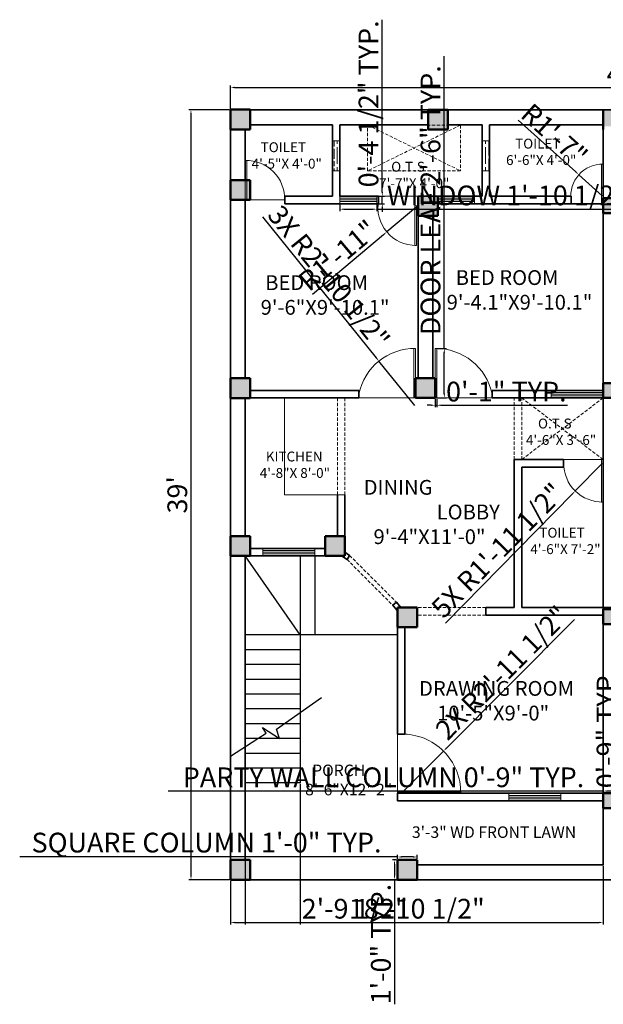
# Model space of a CAD drawing. Units: inches. Extents: x 2499 to 3266, y 1908 to 2597.
# Tile 1 of 2: x 2499 to 2854, y 1908 to 2507. Entities that reach past the tile are written whole.
import ezdxf

# ---------------------------------------------------------------- set-up
doc = ezdxf.new("R2010")
doc.units = ezdxf.units.IN
doc.linetypes.add('JIS_02_2.0', pattern=[3, 2, -1])
for name, color, linetype, lineweight in [('A-ANNO-DIMS', 2, 'Continuous', 18), ('A-AREA-IDEN', 7, 'Continuous', 18), ('A-COLS', 7, 'Continuous', 50), ('A-FLOR-FIXT', 9, 'Continuous', 18), ('A-FLOR-OPEN', 6, 'JIS_02_2.0', 13), ('A-FLOR-STRS', 7, 'Continuous', 25), ('A-GLAZ', 5, 'Continuous', 18), ('A-GLAZ-PATT', 4, 'Continuous', 13), ('A-WALL', 7, 'Continuous', 35), ('A-WALL-OVHD', 6, 'JIS_02_2.0', 18)]:
    doc.layers.add(name, color=color, linetype=linetype, lineweight=lineweight)
doc.layers.add('A-COLS-PATT', color=177, linetype='Continuous', lineweight=13, true_color=0x293189)
doc.layers.add('A-DOOR', color=32, linetype='Continuous', lineweight=18, true_color=0xcd6928)
doc.styles.get("Standard").update_dxf_attribs({"font": 'arial.ttf'})
doc.dimstyles.new('ISO-25', dxfattribs={"dimtxt": 12, "dimasz": 2.5, "dimexe": 1.25, "dimexo": 0.625, "dimtad": 1, "dimdec": 1, "dimlunit": 3, "dimtxsty": 'Standard', "dimcen": 2.5, "dimadec": 0, "dimazin": 0, "dimtfac": 1, "dimtdec": 1, "dimtmove": 0, "dimatfit": 3, "dimfxl": 1, "dimarcsym": 0})

# ---------------------------------------------------------------- blocks, each defined once
blk = doc.blocks.new('*D4')
at = {"layer": 'A-ANNO-DIMS', "color": 0, "lineweight": -2, "transparency": 16777216}
for p, q in [((2627.06, 2452.33), (2627.06, 2466.64)), ((3107.06, 2452.33), (3107.06, 2466.64)), ((2629.56, 2465.39), (3104.56, 2465.39))]:
    blk.add_line(p, q, dxfattribs=at)
at = {"layer": 'A-ANNO-DIMS', "color": 0, "transparency": 16777216}
for points in [[(2629.56, 2465.81), (2629.56, 2464.98), (2627.06, 2465.39)], [(3104.56, 2465.81), (3104.56, 2464.98), (3107.06, 2465.39)]]:
    blk.add_solid(points, dxfattribs=at)
at = {"layer": 'Defpoints', "color": 0, "transparency": 16777216}
for p in [(3107.06, 2465.39), (2627.06, 2451.71), (3107.06, 2451.71)]:
    blk.add_point(p, dxfattribs=at)
at = {"layer": 'A-ANNO-DIMS', "color": 0, "transparency": 16777216, "insert": (2867.06, 2472.14), "char_height": 12, "attachment_point": 5}
blk.add_mtext("40'", dxfattribs=at)
blk = doc.blocks.new('*D5')
at = {"layer": 'A-ANNO-DIMS', "color": 0, "lineweight": -2, "transparency": 16777216}
for p, q in [((2626.43, 2451.71), (2601.81, 2451.71)), ((2603.06, 2449.21), (2603.06, 1986.21)), ((2626.43, 1983.71), (2601.81, 1983.71))]:
    blk.add_line(p, q, dxfattribs=at)
at = {"layer": 'A-ANNO-DIMS', "color": 0, "transparency": 16777216}
for points in [[(2602.64, 2449.21), (2603.48, 2449.21), (2603.06, 2451.71)], [(2602.64, 1986.21), (2603.48, 1986.21), (2603.06, 1983.71)]]:
    blk.add_solid(points, dxfattribs=at)
at = {"layer": 'Defpoints', "color": 0, "transparency": 16777216}
for p in [(2627.06, 2451.71), (2603.06, 1983.71), (2627.06, 1983.71)]:
    blk.add_point(p, dxfattribs=at)
at = {"layer": 'A-ANNO-DIMS', "color": 0, "transparency": 16777216, "insert": (2596.3, 2217.71), "char_height": 12, "attachment_point": 5, "rotation": 90}
blk.add_mtext("39'", dxfattribs=at)
blk = doc.blocks.new('COL-12X12')
for p, q in [((0, 12), (12, 12)), ((0, 0), (0, 12)), ((12, 12), (12, 0)), ((12, 0), (0, 0))]:
    blk.add_line(p, q)
blk = doc.blocks.new('COL-9X9')
for p, q in [((0, 9), (9, 9)), ((0, 0), (0, 9)), ((9, 9), (9, 0)), ((9, 0), (0, 0))]:
    blk.add_line(p, q)
blk = doc.blocks.new('WIN-31_54')
for p, q in [((0, 4.5), (0, 0)), ((0, 3.25), (31.54, 3.25)), ((0, 2.25), (31.54, 2.25)), ((0, 1.25), (31.54, 1.25)), ((31.54, 0), (31.54, 4.5)), ((31.54, 3.25), (31.54, 0))]:
    blk.add_line(p, q)
blk = doc.blocks.new('WIN-22_41')
for p, q in [((0, 4.5), (0, 0)), ((22.41, 3.25), (0, 3.25)), ((22.41, 2.25), (0, 2.25)), ((22.41, 1.25), (0, 1.25)), ((22.41, 4.5), (22.41, 0))]:
    blk.add_line(p, q)
blk = doc.blocks.new('STAIR-BREAK')
for p, q in [((28.01, 16.3), (55.25, 35.7)), ((16.69, 10.65), (21.73, 13.87)), ((21.73, 13.87), (19.46, 17.43)), ((19.46, 17.43), (29.77, 10.65)), ((29.77, 10.65), (28.01, 16.3)), ((0, 0), (16.69, 10.65))]:
    blk.add_line(p, q)
blk = doc.blocks.new('OTS-REAR-OPENING')
for p, q in [((0, 27.82), (56.41, 0)), ((56.41, 27.82), (0, 0))]:
    blk.add_line(p, q)
blk.add_lwpolyline([(0, 27.82), (56.41, 27.82), (56.41, 0), (0, 0)], close=True)
blk = doc.blocks.new('DOOR-LEAF-24')
for p, q in [((0, 0), (0, 24)), ((0, 24), (1, 24)), ((1, 24), (1, 0)), ((1, 0), (0, 0))]:
    blk.add_line(p, q)
blk = doc.blocks.new('DOOR-LEAF-30')
for p, q in [((0, 6), (0, 30)), ((0, 30), (1, 30)), ((1, 30), (1, 0)), ((1, 0), (0, 0))]:
    blk.add_line(p, q)
blk = doc.blocks.new('*D14')
at = {"layer": 'A-ANNO-DIMS', "color": 0, "lineweight": -2, "transparency": 16777216}
for p, q in [((2728.56, 1997.51), (2498.96, 1997.51)), ((2728.56, 1996.33), (2728.56, 1998.76)), ((2738.06, 1997.51), (2731.06, 1997.51)), ((2740.56, 1996.33), (2740.56, 1998.76))]:
    blk.add_line(p, q, dxfattribs=at)
at = {"layer": 'A-ANNO-DIMS', "color": 0, "transparency": 16777216}
for points in [[(2731.06, 1997.93), (2731.06, 1997.09), (2728.56, 1997.51)], [(2738.06, 1997.93), (2738.06, 1997.09), (2740.56, 1997.51)]]:
    blk.add_solid(points, dxfattribs=at)
at = {"layer": 'Defpoints', "color": 0, "transparency": 16777216}
for p in [(2728.56, 1997.51), (2728.56, 1995.71), (2740.56, 1995.71)]:
    blk.add_point(p, dxfattribs=at)
at = {"layer": 'A-ANNO-DIMS', "color": 0, "transparency": 16777216, "insert": (2612.51, 2004.71), "char_height": 12, "attachment_point": 5}
blk.add_mtext('SQUARE COLUMN 1\'-0" TYP.', dxfattribs=at)
blk = doc.blocks.new('*D15')
at = {"layer": 'A-ANNO-DIMS', "color": 0, "lineweight": -2, "transparency": 16777216}
for p, q in [((2727.93, 1995.71), (2725.51, 1995.71)), ((2726.76, 1993.21), (2726.76, 1986.21)), ((2727.93, 1983.71), (2725.51, 1983.71)), ((2726.76, 1983.71), (2726.76, 1907.94))]:
    blk.add_line(p, q, dxfattribs=at)
at = {"layer": 'A-ANNO-DIMS', "color": 0, "transparency": 16777216}
for points in [[(2726.34, 1993.21), (2727.17, 1993.21), (2726.76, 1995.71)], [(2726.34, 1986.21), (2727.17, 1986.21), (2726.76, 1983.71)]]:
    blk.add_solid(points, dxfattribs=at)
at = {"layer": 'Defpoints', "color": 0, "transparency": 16777216}
for p in [(2728.56, 1995.71), (2726.76, 1983.71), (2728.56, 1983.71)]:
    blk.add_point(p, dxfattribs=at)
at = {"layer": 'A-ANNO-DIMS', "color": 0, "transparency": 16777216, "insert": (2720.01, 1944.58), "char_height": 12, "attachment_point": 5, "rotation": 90}
blk.add_mtext('1\'-0" TYP.', dxfattribs=at)
blk = doc.blocks.new('*D16')
at = {"layer": 'A-ANNO-DIMS', "color": 0, "lineweight": -2, "transparency": 16777216}
for p, q in [((2853.56, 2037.57), (2589.1, 2037.57)), ((2853.56, 2036.85), (2853.56, 2038.82)), ((2860.06, 2037.57), (2856.06, 2037.57)), ((2862.56, 2036.85), (2862.56, 2038.82))]:
    blk.add_line(p, q, dxfattribs=at)
at = {"layer": 'A-ANNO-DIMS', "color": 0, "transparency": 16777216}
for points in [[(2856.06, 2037.99), (2856.06, 2037.15), (2853.56, 2037.57)], [(2860.06, 2037.99), (2860.06, 2037.15), (2862.56, 2037.57)]]:
    blk.add_solid(points, dxfattribs=at)
at = {"layer": 'Defpoints', "color": 0, "transparency": 16777216}
for p in [(2853.56, 2037.57), (2853.56, 2036.22), (2862.56, 2036.22)]:
    blk.add_point(p, dxfattribs=at)
at = {"layer": 'A-ANNO-DIMS', "color": 0, "transparency": 16777216, "insert": (2720.08, 2044.4), "char_height": 12, "attachment_point": 5}
blk.add_mtext('PARTY WALL COLUMN 0\'-9" TYP.', dxfattribs=at)
blk = doc.blocks.new('*D17')
at = {"layer": 'A-ANNO-DIMS', "color": 0, "lineweight": -2, "transparency": 16777216}
for p, q in [((2863.91, 2036.22), (2863.91, 2113.12)), ((2863.18, 2036.22), (2865.16, 2036.22)), ((2863.91, 2029.72), (2863.91, 2033.72)), ((2863.18, 2027.22), (2865.16, 2027.22))]:
    blk.add_line(p, q, dxfattribs=at)
at = {"layer": 'A-ANNO-DIMS', "color": 0, "transparency": 16777216}
for points in [[(2863.49, 2033.72), (2864.32, 2033.72), (2863.91, 2036.22)], [(2863.49, 2029.72), (2864.32, 2029.72), (2863.91, 2027.22)]]:
    blk.add_solid(points, dxfattribs=at)
at = {"layer": 'Defpoints', "color": 0, "transparency": 16777216}
for p in [(2862.56, 2036.22), (2863.91, 2036.22), (2862.56, 2027.22)]:
    blk.add_point(p, dxfattribs=at)
at = {"layer": 'A-ANNO-DIMS', "color": 0, "transparency": 16777216, "insert": (2857.16, 2075.92), "char_height": 12, "attachment_point": 5, "rotation": 90}
blk.add_mtext('0\'-9" TYP.', dxfattribs=at)
blk = doc.blocks.new('*D20')
at = {"layer": 'A-ANNO-DIMS', "color": 0, "lineweight": -2, "transparency": 16777216}
for p, q in [((2693.56, 2394.08), (2693.56, 2390.1)), ((2696.06, 2391.35), (2713.47, 2391.35)), ((2715.97, 2394.08), (2715.97, 2390.1)), ((2715.97, 2391.35), (2908.86, 2391.35))]:
    blk.add_line(p, q, dxfattribs=at)
at = {"layer": 'A-ANNO-DIMS', "color": 0, "transparency": 16777216}
for points in [[(2696.06, 2391.76), (2696.06, 2390.93), (2693.56, 2391.35)], [(2713.47, 2391.76), (2713.47, 2390.93), (2715.97, 2391.35)]]:
    blk.add_solid(points, dxfattribs=at)
at = {"layer": 'Defpoints', "color": 0, "transparency": 16777216}
for p in [(2693.56, 2394.71), (2715.97, 2394.71), (2715.97, 2391.35)]:
    blk.add_point(p, dxfattribs=at)
at = {"layer": 'A-ANNO-DIMS', "color": 0, "transparency": 16777216, "insert": (2813.66, 2398.18), "char_height": 12, "attachment_point": 5}
blk.add_mtext('WINDOW 1\'-10 1/2" TYP.', dxfattribs=at)
blk = doc.blocks.new('*D21')
at = {"layer": 'A-ANNO-DIMS', "color": 0, "lineweight": -2, "transparency": 16777216}
for p, q in [((2719.33, 2401.71), (2719.33, 2506.57)), ((2716.6, 2399.21), (2720.58, 2399.21)), ((2716.6, 2394.71), (2720.58, 2394.71)), ((2719.33, 2394.71), (2719.33, 2399.21)), ((2719.33, 2392.21), (2719.33, 2389.71))]:
    blk.add_line(p, q, dxfattribs=at)
at = {"layer": 'A-ANNO-DIMS', "color": 0, "transparency": 16777216}
for points in [[(2718.92, 2401.71), (2719.75, 2401.71), (2719.33, 2399.21)], [(2718.92, 2392.21), (2719.75, 2392.21), (2719.33, 2394.71)]]:
    blk.add_solid(points, dxfattribs=at)
at = {"layer": 'Defpoints', "color": 0, "transparency": 16777216}
for p in [(2715.97, 2399.21), (2715.97, 2394.71), (2719.33, 2399.21)]:
    blk.add_point(p, dxfattribs=at)
at = {"layer": 'A-ANNO-DIMS', "color": 0, "transparency": 16777216, "insert": (2712.5, 2455.39), "char_height": 12, "attachment_point": 5, "rotation": 90}
blk.add_mtext('0\'-4 1/2" TYP.', dxfattribs=at)
blk = doc.blocks.new('*D24')
at = {"layer": 'A-ANNO-DIMS', "color": 0, "lineweight": -2, "transparency": 16777216}
for p, q in [((2757.02, 2306.66), (2757.02, 2484.49)), ((2753.15, 2306.66), (2758.27, 2306.66)), ((2757.02, 2279.16), (2757.02, 2304.16)), ((2753.15, 2276.66), (2758.27, 2276.66))]:
    blk.add_line(p, q, dxfattribs=at)
at = {"layer": 'A-ANNO-DIMS', "color": 0, "transparency": 16777216}
for points in [[(2756.6, 2304.16), (2757.44, 2304.16), (2757.02, 2306.66)], [(2756.6, 2279.16), (2757.44, 2279.16), (2757.02, 2276.66)]]:
    blk.add_solid(points, dxfattribs=at)
at = {"layer": 'Defpoints', "color": 0, "transparency": 16777216}
for p in [(2752.52, 2306.66), (2757.02, 2306.66), (2752.52, 2276.66)]:
    blk.add_point(p, dxfattribs=at)
at = {"layer": 'A-ANNO-DIMS', "color": 0, "transparency": 16777216, "insert": (2750.19, 2396.83), "char_height": 12, "attachment_point": 5, "rotation": 90}
blk.add_mtext('DOOR LEAF 2\'-6" TYP.', dxfattribs=at)
blk = doc.blocks.new('*D25')
at = {"layer": 'A-ANNO-DIMS', "color": 0, "lineweight": -2, "transparency": 16777216}
for p, q in [((2751.52, 2276.04), (2751.52, 2270.91)), ((2752.52, 2276.04), (2752.52, 2270.91)), ((2749.02, 2272.16), (2746.52, 2272.16)), ((2751.52, 2272.16), (2752.52, 2272.16)), ((2755.02, 2272.16), (2831.92, 2272.16))]:
    blk.add_line(p, q, dxfattribs=at)
at = {"layer": 'A-ANNO-DIMS', "color": 0, "transparency": 16777216}
for points in [[(2749.02, 2272.58), (2749.02, 2271.75), (2751.52, 2272.16)], [(2755.02, 2272.58), (2755.02, 2271.75), (2752.52, 2272.16)]]:
    blk.add_solid(points, dxfattribs=at)
at = {"layer": 'Defpoints', "color": 0, "transparency": 16777216}
for p in [(2751.52, 2276.66), (2752.52, 2276.66), (2752.52, 2272.16)]:
    blk.add_point(p, dxfattribs=at)
at = {"layer": 'A-ANNO-DIMS', "color": 0, "transparency": 16777216, "insert": (2794.72, 2278.91), "char_height": 12, "attachment_point": 5}
blk.add_mtext('0\'-1" TYP.', dxfattribs=at)
blk = doc.blocks.new('*D28')
at = {"layer": 'A-ANNO-DIMS', "color": 0, "lineweight": -2, "transparency": 16777216}
for p, q in [((2853.56, 1992.08), (2853.56, 1956.43)), ((2627.06, 1983.08), (2627.06, 1956.43)), ((2629.56, 1957.68), (2851.06, 1957.68))]:
    blk.add_line(p, q, dxfattribs=at)
at = {"layer": 'A-ANNO-DIMS', "color": 0, "transparency": 16777216}
for points in [[(2629.56, 1958.1), (2629.56, 1957.27), (2627.06, 1957.68)], [(2851.06, 1958.1), (2851.06, 1957.27), (2853.56, 1957.68)]]:
    blk.add_solid(points, dxfattribs=at)
at = {"layer": 'Defpoints', "color": 0, "transparency": 16777216}
for p in [(2853.56, 1992.71), (2627.06, 1983.71), (2853.56, 1957.68)]:
    blk.add_point(p, dxfattribs=at)
at = {"layer": 'A-ANNO-DIMS', "color": 0, "transparency": 16777216, "insert": (2740.31, 1964.51), "char_height": 12, "attachment_point": 5}
blk.add_mtext('18\'-10 1/2"', dxfattribs=at)
blk = doc.blocks.new('*D31')
at = {"layer": 'A-ANNO-DIMS', "color": 0, "lineweight": -2, "transparency": 16777216}
for p, q in [((2636.06, 2041.89), (2636.06, 1956.43)), ((2669.43, 2041.89), (2669.43, 1956.43)), ((2638.56, 1957.68), (2666.93, 1957.68)), ((2669.43, 1957.68), (2733.24, 1957.68))]:
    blk.add_line(p, q, dxfattribs=at)
at = {"layer": 'A-ANNO-DIMS', "color": 0, "transparency": 16777216}
for points in [[(2638.56, 1958.1), (2638.56, 1957.27), (2636.06, 1957.68)], [(2666.93, 1958.1), (2666.93, 1957.27), (2669.43, 1957.68)]]:
    blk.add_solid(points, dxfattribs=at)
at = {"layer": 'Defpoints', "color": 0, "transparency": 16777216}
for p in [(2636.06, 2042.51), (2669.43, 2042.51), (2669.43, 1957.68)]:
    blk.add_point(p, dxfattribs=at)
at = {"layer": 'A-ANNO-DIMS', "color": 0, "transparency": 16777216, "insert": (2702.58, 1964.51), "char_height": 12, "attachment_point": 5}
blk.add_mtext('2\'-9 1/2"', dxfattribs=at)
blk = doc.blocks.new('*D34')
at = {"layer": 'A-ANNO-DIMS', "color": 0, "lineweight": -2, "transparency": 16777216}
for p, q in [((2836.17, 2141.9), (2758.28, 2063.65)), ((2731.47, 2036.71), (2756.52, 2061.87))]:
    blk.add_line(p, q, dxfattribs=at)
at = {"layer": 'A-ANNO-DIMS', "color": 0, "transparency": 16777216}
blk.add_solid([(2757.99, 2063.94), (2758.58, 2063.35), (2756.52, 2061.87)], dxfattribs=at)
at = {"layer": 'Defpoints', "color": 0, "transparency": 16777216}
for p in [(2756.52, 2061.87), (2731.47, 2036.71)]:
    blk.add_point(p, dxfattribs=at)
at = {"layer": 'A-ANNO-DIMS', "color": 0, "transparency": 16777216, "insert": (2793.27, 2108.48), "char_height": 12, "attachment_point": 5, "rotation": 45.13418}
blk.add_mtext('2X R2\'-11 1/2"', dxfattribs=at)
blk = doc.blocks.new('*D36')
at = {"layer": 'A-ANNO-DIMS', "color": 0, "lineweight": -2, "transparency": 16777216}
for p, q in [((2646.51, 2386.7), (2715.7, 2300.93)), ((2739.02, 2272.02), (2717.27, 2298.99))]:
    blk.add_line(p, q, dxfattribs=at)
at = {"layer": 'A-ANNO-DIMS', "color": 0, "transparency": 16777216}
blk.add_solid([(2716.02, 2301.19), (2715.37, 2300.67), (2717.27, 2298.99)], dxfattribs=at)
at = {"layer": 'Defpoints', "color": 0, "transparency": 16777216}
for p in [(2717.27, 2298.99), (2739.02, 2272.02)]:
    blk.add_point(p, dxfattribs=at)
at = {"layer": 'A-ANNO-DIMS', "color": 0, "transparency": 16777216, "insert": (2685.64, 2349.08), "char_height": 12, "attachment_point": 5, "rotation": 308.89333}
blk.add_mtext('3X R2\'-10 1/2"', dxfattribs=at)
blk = doc.blocks.new('*D37')
at = {"layer": 'A-ANNO-DIMS', "color": 0, "lineweight": -2, "transparency": 16777216}
for p, q in [((2853.06, 2236.82), (2836.6, 2220.04)), ((2757.7, 2139.57), (2834.85, 2218.26))]:
    blk.add_line(p, q, dxfattribs=at)
at = {"layer": 'A-ANNO-DIMS', "color": 0, "transparency": 16777216}
blk.add_solid([(2834.56, 2218.55), (2835.15, 2217.96), (2836.6, 2220.04)], dxfattribs=at)
at = {"layer": 'Defpoints', "color": 0, "transparency": 16777216}
for p in [(2853.06, 2236.82), (2836.6, 2220.04)]:
    blk.add_point(p, dxfattribs=at)
at = {"layer": 'A-ANNO-DIMS', "color": 0, "transparency": 16777216, "insert": (2790.52, 2182.8), "char_height": 12, "attachment_point": 5, "rotation": 45.56344}
blk.add_mtext('5X R1\'-11 1/2"', dxfattribs=at)
blk = doc.blocks.new('*D38')
at = {"layer": 'A-ANNO-DIMS', "color": 0, "lineweight": -2, "transparency": 16777216}
for p, q in [((2739.74, 2392.38), (2722.06, 2377.53)), ((2676.92, 2339.61), (2720.15, 2375.92))]:
    blk.add_line(p, q, dxfattribs=at)
at = {"layer": 'A-ANNO-DIMS', "color": 0, "transparency": 16777216}
blk.add_solid([(2719.88, 2376.24), (2720.42, 2375.6), (2722.06, 2377.53)], dxfattribs=at)
at = {"layer": 'Defpoints', "color": 0, "transparency": 16777216}
for p in [(2739.74, 2392.38), (2722.06, 2377.53)]:
    blk.add_point(p, dxfattribs=at)
at = {"layer": 'A-ANNO-DIMS', "color": 0, "transparency": 16777216, "insert": (2693.3, 2362.05), "char_height": 12, "attachment_point": 5, "rotation": 40.03317}
blk.add_mtext('R1\'-11"', dxfattribs=at)
blk = doc.blocks.new('*D40')
at = {"layer": 'A-ANNO-DIMS', "color": 0, "lineweight": -2, "transparency": 16777216}
for p, q in [((2801.82, 2445.47), (2836.92, 2414.01)), ((2853.06, 2399.54), (2838.78, 2412.34))]:
    blk.add_line(p, q, dxfattribs=at)
at = {"layer": 'A-ANNO-DIMS', "color": 0, "transparency": 16777216}
blk.add_solid([(2837.2, 2414.32), (2836.64, 2413.7), (2838.78, 2412.34)], dxfattribs=at)
at = {"layer": 'Defpoints', "color": 0, "transparency": 16777216}
for p in [(2838.78, 2412.34), (2853.06, 2399.54)]:
    blk.add_point(p, dxfattribs=at)
at = {"layer": 'A-ANNO-DIMS', "color": 0, "transparency": 16777216, "insert": (2822.88, 2435.53), "char_height": 12, "attachment_point": 5, "rotation": 318.12284}
blk.add_mtext('R1\'-7"', dxfattribs=at)

msp = doc.modelspace()

# ---------------------------------------------------------------- hatches: boundary and pattern name
at = {"layer": 'A-COLS-PATT'}
h = msp.add_hatch(color=256, dxfattribs=at)
h.dxf.hatch_style = 1
h.paths.add_polyline_path([(2639.06, 2451.71), (2627.06, 2451.71), (2627.06, 2439.9), (2639.06, 2439.9)])
h.paths.add_polyline_path([(2639.06, 2408.96), (2627.06, 2408.96), (2627.06, 2396.96), (2639.06, 2396.96)])
h.paths.add_polyline_path([(2759.22, 2451.71), (2747.22, 2451.71), (2747.22, 2439.71), (2759.22, 2439.71)])
h.paths.add_polyline_path([(2862.56, 2451.71), (2853.74, 2451.71), (2853.56, 2451.71), (2853.56, 2441.73), (2853.74, 2441.73), (2853.74, 2441.73), (2862.56, 2441.73), (2862.56, 2442.71)])
h.paths.add_polyline_path([(2989.26, 2451.71), (2977.26, 2451.71), (2977.26, 2439.71), (2989.26, 2439.71)])
h.paths.add_polyline_path([(3107.06, 2451.71), (3095.06, 2451.71), (3095.06, 2439.71), (3107.06, 2439.71)])
h.paths.add_polyline_path([(3107.06, 2399.21), (3095.06, 2399.21), (3095.06, 2387.21), (3107.06, 2387.21)])
h.paths.add_polyline_path([(2989.26, 2399.21), (2977.26, 2399.21), (2977.26, 2387.21), (2989.26, 2387.21)])
h.paths.add_polyline_path([(2862.56, 2397.96), (2853.56, 2397.96), (2853.56, 2388.96), (2862.56, 2388.96)])
h.paths.add_polyline_path([(2753.06, 2399.21), (2741.06, 2399.21), (2741.06, 2387.39), (2753.06, 2387.39)])
h.paths.add_polyline_path([(2639.06, 2288.56), (2627.06, 2288.56), (2627.06, 2276.56), (2636.06, 2276.56), (2636.06, 2276.61), (2639.06, 2276.61)])
h.paths.add_polyline_path([(2862.56, 2285.61), (2853.56, 2285.61), (2853.56, 2276.61), (2862.56, 2276.61)])
h.paths.add_polyline_path([(2990.61, 2288.63), (2978.61, 2288.63), (2978.61, 2276.63), (2990.61, 2276.63)])
h.paths.add_polyline_path([(3107.06, 2288.61), (3095.06, 2288.61), (3095.06, 2276.61), (3107.06, 2276.61)])
h.paths.add_polyline_path([(3107.06, 2192.61), (3095.06, 2192.61), (3095.06, 2180.61), (3107.06, 2180.61)])
h.paths.add_polyline_path([(3045.56, 2192.61), (3033.56, 2192.61), (3033.56, 2180.61), (3045.56, 2180.61)])
h.paths.add_polyline_path([(2639.06, 2192.61), (2627.06, 2192.61), (2627.06, 2180.61), (2639.06, 2180.61)])
h.paths.add_polyline_path([(2696.54, 2192.61), (2684.54, 2192.61), (2684.54, 2180.61), (2696.54, 2180.61)])
h.paths.add_polyline_path([(2740.56, 2149.11), (2728.56, 2149.11), (2728.56, 2137.17), (2740.56, 2137.17)])
h.paths.add_polyline_path([(2862.56, 2148.12), (2853.56, 2148.12), (2853.56, 2139.12), (2862.56, 2139.12)])
h.paths.add_polyline_path([(2987.56, 2149.11), (2975.54, 2149.11), (2975.54, 2137.05), (2987.56, 2137.05)])
h.paths.add_polyline_path([(2862.56, 2036.21), (2853.56, 2036.21), (2853.56, 2027.22), (2862.56, 2027.22)])
h.paths.add_polyline_path([(2639.06, 1995.71), (2627.06, 1995.71), (2627.06, 1983.71), (2639.06, 1983.71)])
h.paths.add_polyline_path([(2740.56, 1995.71), (2728.56, 1995.71), (2728.56, 1983.71), (2740.56, 1983.71)])
h.paths.add_polyline_path([(2987.56, 1995.71), (2975.56, 1995.71), (2975.56, 1983.71), (2987.56, 1983.71)])
h.paths.add_polyline_path([(3107.06, 1995.71), (3095.06, 1995.71), (3095.06, 1983.71), (3107.06, 1983.71)])
h = msp.add_hatch(color=256, dxfattribs=at)
h.dxf.hatch_style = 1
h.paths.add_polyline_path([(2751.52, 2288.66), (2739.52, 2288.66), (2739.52, 2276.66), (2751.52, 2276.66)])
at = {"layer": 'A-GLAZ-PATT'}
h = msp.add_hatch(dxfattribs=at)
h.set_pattern_fill('GOST_WOOD', color=256)
h.paths.add_polyline_path([(2693.56, 2432.95), (2689.06, 2432.95), (2689.06, 2414.75), (2693.56, 2414.75)])
h.paths.add_polyline_path([(2784.56, 2432.95), (2780.06, 2432.95), (2780.06, 2414.75), (2784.56, 2414.75)])
h.paths.add_polyline_path([(2940.56, 2432.95), (2936.06, 2432.95), (2936.06, 2414.75), (2940.56, 2414.75)])
h.paths.add_polyline_path([(3031.56, 2432.95), (3027.06, 2432.95), (3027.06, 2414.75), (3031.56, 2414.75)])

# ---------------------------------------------------------------- linework, layer by layer
at = {"layer": 'A-COLS'}
for p, q in [((2853.56, 2439.71), (2853.56, 2451.71)), ((2853.74, 2441.73), (2853.56, 2441.73)), ((2741.06, 2387.39), (2741.06, 2399.21)), ((2753.06, 2399.21), (2753.06, 2387.39)), ((2753.06, 2387.39), (2741.06, 2387.39)), ((2636.06, 2180.61), (2627.06, 2180.61)), ((2728.56, 2149.11), (2740.56, 2149.11)), ((2728.56, 2137.17), (2728.56, 2149.11)), ((2740.56, 2149.11), (2740.56, 2137.17)), ((2740.56, 2137.17), (2728.56, 2137.17)), ((2728.56, 1995.71), (2728.56, 1983.71))]:
    msp.add_line(p, q, dxfattribs=at)
at = {"layer": 'A-DOOR'}
for p, q in [((2636.06, 2396.96), (2636.06, 2420.96)), ((2636.06, 2420.96), (2637.06, 2420.96)), ((2637.06, 2420.96), (2637.06, 2396.96)), ((2660.06, 2396.96), (2636.06, 2396.96)), ((2717.06, 2399.21), (2741.06, 2399.21)), ((2834.06, 2394.71), (2852.56, 2394.71)), ((2741.06, 2393.3), (2740.06, 2393.3)), ((2739.52, 2306.66), (2738.52, 2306.66)), ((2738.52, 2306.66), (2738.57, 2276.66)), ((2739.52, 2282.66), (2739.52, 2306.66)), ((2738.52, 2276.66), (2705.06, 2276.61)), ((2738.52, 2276.66), (2739.52, 2276.66)), ((2752.52, 2276.66), (2786.06, 2276.61)), ((2853.56, 2239.11), (2829.56, 2239.11)), ((2852.56, 2213.33), (2852.56, 2239.11)), ((2852.56, 2239.11), (2853.56, 2239.11)), ((2853.56, 2237.33), (2853.56, 2213.33)), ((2853.56, 2213.33), (2852.56, 2213.33)), ((2728.56, 2036.21), (2728.56, 2072.21)), ((2730.98, 2037.21), (2728.56, 2037.21)), ((2728.56, 2037.21), (2728.56, 2036.21)), ((2754.98, 2037.21), (2730.98, 2037.21)), ((2730.98, 2036.21), (2754.98, 2036.21)), ((2754.98, 2036.21), (2754.98, 2037.21)), ((2766.98, 2037.21), (2754.98, 2037.21)), ((2754.98, 2036.21), (2766.98, 2036.21)), ((2766.98, 2036.21), (2766.98, 2037.21))]:
    msp.add_line(p, q, dxfattribs=at)
for centre, radius, start, end in [((2636.56, 2397.46), 23.51, 358.78112, 91.21888), ((2853.06, 2399.54), 19.17, 88.50578, 187.73848), ((2739.74, 2392.38), 23.08, 169.27414, 270.79204), ((2739.02, 2272.02), 34.65, 89.1731, 168.61507), ((2752.02, 2271.93), 34.73, 11.50222, 90.82483), ((2853.06, 2236.82), 23.5, 179.90805, 271.21915), ((2731.47, 2036.71), 35.51, 359.19313, 91.07497)]:
    msp.add_arc(centre, radius, start, end, dxfattribs=at)
at = {"layer": 'A-FLOR-FIXT'}
for p, q in [((2659.83, 2217.63), (2659.83, 2276.61)), ((2696.56, 2217.63), (2659.83, 2217.63))]:
    msp.add_line(p, q, dxfattribs=at)
at = {"layer": 'A-FLOR-OPEN'}
for p, q in [((2710.42, 2414.75), (2710.56, 2414.75)), ((2766.7, 2414.75), (2766.84, 2414.75)), ((2799.56, 2239.11), (2799.56, 2276.61)), ((2804.06, 2239.11), (2804.06, 2276.61)), ((2853.56, 2276.61), (2804.06, 2239.11)), ((2804.06, 2239.11), (2804.06, 2276.61)), ((2804.06, 2276.61), (2853.56, 2239.11))]:
    msp.add_line(p, q, dxfattribs=at)
at = {"layer": 'A-FLOR-STRS'}
for p, q in [((2669.43, 2132.51), (2636.06, 2180.61)), ((2669.43, 2180.61), (2669.43, 2042.51)), ((2678.43, 2180.61), (2678.43, 2132.51)), ((2728.56, 2132.51), (2636.06, 2132.51)), ((2669.43, 2132.51), (2669.43, 2123.51)), ((2669.43, 2123.51), (2636.06, 2123.51)), ((2669.43, 2114.51), (2636.06, 2114.51)), ((2669.43, 2105.51), (2636.06, 2105.51)), ((2669.43, 2096.51), (2636.06, 2096.51)), ((2669.43, 2087.51), (2636.06, 2087.51)), ((2669.43, 2078.51), (2636.06, 2078.51)), ((2669.43, 2069.51), (2636.06, 2069.51)), ((2669.43, 2060.51), (2636.06, 2060.51)), ((2669.43, 2051.51), (2636.06, 2051.51)), ((2669.43, 2042.51), (2636.06, 2042.51))]:
    msp.add_line(p, q, dxfattribs=at)
at = {"layer": 'A-GLAZ'}
for p, q in [((2689.06, 2432.95), (2693.56, 2432.95)), ((2689.06, 2414.75), (2689.06, 2432.95)), ((2693.56, 2432.95), (2693.56, 2414.75)), ((2780.06, 2432.95), (2784.56, 2432.95)), ((2693.56, 2414.75), (2689.06, 2414.75)), ((2780.06, 2414.75), (2784.56, 2414.75)), ((2822.02, 2281.11), (2822.02, 2276.61)), ((2822.02, 2279.86), (2853.56, 2279.86)), ((2822.02, 2278.86), (2853.56, 2278.86)), ((2822.02, 2277.86), (2853.56, 2277.86))]:
    msp.add_line(p, q, dxfattribs=at)
at = {"layer": 'A-WALL'}
for p, q in [((2627.06, 2451.71), (3107.06, 2451.71)), ((2627.06, 1983.71), (2627.06, 2451.71)), ((2639.06, 2442.71), (2689.06, 2442.71)), ((2689.06, 2399.21), (2689.06, 2442.71)), ((2693.56, 2399.21), (2693.56, 2442.71)), ((2693.56, 2442.71), (2747.22, 2442.71)), ((2759.22, 2442.71), (2780.06, 2442.71)), ((2780.06, 2399.21), (2780.06, 2442.71)), ((2784.56, 2399.21), (2784.56, 2442.71)), ((2784.56, 2442.71), (2853.56, 2442.71)), ((2853.56, 1992.71), (2853.56, 2442.71)), ((2636.06, 2408.96), (2636.06, 2439.9)), ((2636.06, 2288.56), (2636.06, 2396.96)), ((2660.06, 2399.21), (2689.06, 2399.21)), ((2660.06, 2394.71), (2660.06, 2399.21)), ((2660.06, 2394.71), (2717.06, 2394.71)), ((2693.56, 2399.21), (2717.06, 2399.21)), ((2717.06, 2399.21), (2717.06, 2394.71)), ((2741.06, 2399.21), (2780.06, 2399.21)), ((2741.06, 2288.66), (2741.06, 2399.21)), ((2753.06, 2394.71), (2834.06, 2394.71)), ((2784.56, 2399.21), (2834.06, 2399.21)), ((2834.06, 2394.71), (2834.06, 2399.21)), ((2834.06, 2394.71), (2853.56, 2394.71)), ((2750.06, 2288.66), (2750.06, 2387.39)), ((2639.06, 2281.11), (2705.06, 2281.11)), ((2705.06, 2276.61), (2705.06, 2281.11)), ((2786.06, 2276.61), (2786.06, 2281.11)), ((2786.06, 2281.11), (2853.56, 2281.11)), ((2636.06, 2276.61), (2705.06, 2276.61)), ((2636.06, 2192.61), (2636.06, 2276.61)), ((2786.06, 2276.61), (2944.26, 2276.61)), ((2799.56, 2149.11), (2799.56, 2239.11)), ((2799.56, 2239.11), (2829.56, 2239.11)), ((2829.56, 2239.11), (2829.56, 2234.61)), ((2804.06, 2149.11), (2804.06, 2234.61)), ((2804.06, 2234.61), (2829.56, 2234.61)), ((2692.06, 2192.61), (2692.06, 2217.63)), ((2696.56, 2180.61), (2696.56, 2217.63)), ((2639.06, 2185.11), (2684.54, 2185.11)), ((2696.54, 2185.11), (2696.56, 2185.11)), ((2636.06, 1995.71), (2636.06, 2180.61)), ((2636.06, 2180.61), (2696.56, 2180.61)), ((2696.54, 2180.61), (2694.54, 2180.61)), ((2694.54, 2180.61), (2697.9, 2178.43)), ((2696.54, 2182.77), (2699.47, 2180.87)), ((2696.56, 2180.61), (2696.56, 2182.61)), ((2697.9, 2178.43), (2699.47, 2180.87)), ((2725.65, 2150.57), (2727.9, 2152.39)), ((2728.3, 2147.29), (2725.65, 2150.57)), ((2730.56, 2149.11), (2727.9, 2152.39)), ((2728.56, 2072.21), (2728.56, 2149.11)), ((2728.56, 2149.11), (2730.56, 2149.11)), ((2728.56, 2149.11), (2728.56, 2147.11)), ((2782.16, 2149.11), (2782.16, 2144.61)), ((2782.16, 2149.11), (2799.56, 2149.11)), ((2786.06, 2149.11), (2799.56, 2149.11)), ((2804.06, 2149.11), (2907.56, 2149.11)), ((2804.06, 2149.11), (2907.56, 2149.11)), ((2782.16, 2144.61), (2804.06, 2144.61)), ((2786.06, 2144.61), (2853.56, 2144.61)), ((2804.06, 2144.61), (2853.56, 2144.61)), ((2733.06, 2072.21), (2733.06, 2137.17)), ((2733.06, 2072.21), (2728.56, 2072.21)), ((2728.56, 2031.71), (2728.56, 2036.21)), ((2987.56, 2036.21), (2728.56, 2036.21)), ((2853.56, 2031.71), (2728.56, 2031.71)), ((2853.56, 1992.71), (2740.56, 1992.71)), ((3107.06, 1983.71), (2627.06, 1983.71))]:
    msp.add_line(p, q, dxfattribs=at)
at = {"layer": 'A-WALL-OVHD'}
for p, q in [((2692.06, 2217.63), (2692.06, 2276.61)), ((2696.56, 2217.63), (2696.56, 2276.61)), ((2699.47, 2180.87), (2727.9, 2152.39)), ((2697.9, 2178.43), (2725.65, 2150.57)), ((2782.16, 2149.11), (2740.56, 2149.11)), ((2782.16, 2144.61), (2740.56, 2144.61))]:
    msp.add_line(p, q, dxfattribs=at)

# ---------------------------------------------------------------- block references
at = {"layer": 'A-COLS'}
for name, p, rotation in [('COL-12X12', (2639.06, 2451.9), 180), ('COL-12X12', (2759.22, 2451.71), 180), ('COL-12X12', (2639.06, 2408.96), 180), ('COL-12X12', (2639.06, 2288.56), 180), ('COL-12X12', (2751.52, 2288.66), 180), ('COL-9X9', (2862.56, 2276.61), 89.9999999999884), ('COL-12X12', (2639.06, 2192.61), 180), ('COL-12X12', (2696.54, 2192.61), 180), ('COL-9X9', (2862.56, 2139.12), 89.99999999998552), ('COL-9X9', (2862.56, 2027.22), 89.99999999999422), ('COL-12X12', (2639.06, 1995.71), 180), ('COL-12X12', (2740.56, 1995.71), 180)]:
    msp.add_blockref(name, p, dxfattribs=dict(at, rotation=rotation))
msp.add_blockref('COL-9X9', (2853.56, 2388.96), dxfattribs=at)
at = {"layer": 'A-DOOR'}
for name, p in [('DOOR-LEAF-24', (2852.56, 2394.71)), ('DOOR-LEAF-24', (2739.06, 2369.3)), ('DOOR-LEAF-30', (2751.52, 2276.66))]:
    msp.add_blockref(name, p, dxfattribs=at)
at = {"layer": 'A-FLOR-OPEN'}
msp.add_blockref('OTS-REAR-OPENING', (2710.42, 2414.68), dxfattribs=at)
at = {"layer": 'A-FLOR-STRS'}
msp.add_blockref('STAIR-BREAK', (2627.06, 2058.86), dxfattribs=at)
at = {"layer": 'A-GLAZ'}
for name, p in [('WIN-22_41', (2693.56, 2394.71)), ('WIN-22_41', (2753.06, 2394.71)), ('WIN-31_54', (2646.78, 2180.61)), ('WIN-31_54', (2796.27, 2031.71))]:
    msp.add_blockref(name, p, dxfattribs=at)

# ---------------------------------------------------------------- texts
at = {"layer": 'A-AREA-IDEN', "attachment_point": 1}
for s, width, insert, char_height in [('   TOILET \\P4\'-5"X 4\'-0"', 79.249, (2639.92, 2432.03), 6), ('   TOILET \\P6\'-6"X 4\'-0"', 47.5104, (2794.57, 2434.22), 6), ('    O.T.S \\P7\'-7"X 4\'-0"', 47.5104, (2717.41, 2420.17), 6), ('  BED ROOM\\P9\'-4.1"X9\'-10.1"', 87.691, (2758.44, 2354.28), 9), ('  BED ROOM\\P 9\'-6"X9\'-10.1"', 87.691, (2642.66, 2351.18), 9), ('    O.T.S \\P4\'-6"X 3\'-6"', 47.5104, (2806.64, 2264.04), 6), ('  KITCHEN \\P4\'-8"X 8\'-0"', 44.2597, (2644.87, 2243.99), 6), ('\\pxqc;DINING                                 LOBBY\\P\\pql;   9\'-4"X11\'-0"', 87.691, (2705.74, 2226.74), 9), ('   TOILET \\P4\'-6"X 7\'-2"', 44.2597, (2809.3, 2197.67), 6), ('  DRAWING ROOM\\P      10\'-5"X9\'-0"', 122.0977, (2736.16, 2104.5), 9), ('  PORCH\\P8\'-6"X12\'-2"', 65.76, (2672.43, 2053.66), 7), ('3\'-3" WD FRONT LAWN', 110.856, (2737.34, 2016.11), 7)]:
    msp.add_mtext_dynamic_manual_height_columns(s, width=width, gutter_width=12.5, heights=[0], dxfattribs=dict(at, insert=insert, char_height=char_height))

# ---------------------------------------------------------------- dimensions: what is measured, and where the dimension line sits
at = {"layer": 'A-ANNO-DIMS'}
for base, p1, p2, angle, text, picture, middle in [((2719.33, 2399.21), (2715.97, 2394.71), (2715.97, 2399.21), 90, '<> TYP.', '*D21', (2712.5, 2455.39)), ((2757.02, 2306.66), (2752.52, 2276.66), (2752.52, 2306.66), 90, 'DOOR LEAF <> TYP.', '*D24', (2750.19, 2396.83)), ((2863.91, 2036.22), (2862.56, 2027.22), (2862.56, 2036.22), 90, '<> TYP.', '*D17', (2857.16, 2075.92)), ((2853.56, 2037.57), (2862.56, 2036.22), (2853.56, 2036.22), 180, 'PARTY WALL COLUMN <> TYP.', '*D16', (2720.08, 2044.4)), ((2728.56, 1997.51), (2740.56, 1995.71), (2728.56, 1995.71), 180, 'SQUARE COLUMN <> TYP.', '*D14', (2612.51, 2004.71)), ((2726.76, 1983.71), (2728.56, 1995.71), (2728.56, 1983.71), 270, '<> TYP.', '*D15', (2720.01, 1944.58))]:
    dim = msp.add_linear_dim(base=base, p1=p1, p2=p2, angle=angle, text=text, dimstyle='ISO-25', override={"dimdec": 1, "dimlfac": 1, "dimrnd": 0, "dimzin": 1, "dimdsep": 46, "dimlunit": 4, "dimfrac": 2}, dxfattribs=at)
    dim.commit()
    dim.dimension.update_dxf_attribs({"geometry": picture, "text_midpoint": middle})
for base, p1, p2, override, picture, middle in [((3107.06, 2465.39), (2627.06, 2451.71), (3107.06, 2451.71), {"dimclrd": 0, "dimclre": 0, "dimclrt": 0}, '*D4', (2867.06, 2472.14)), ((2669.43, 1957.68), (2636.06, 2042.51), (2669.43, 2042.51), {"dimdec": 1, "dimlfac": 1, "dimrnd": 0, "dimzin": 1, "dimdsep": 46, "dimlunit": 4, "dimfrac": 2}, '*D31', (2702.58, 1964.51)), ((2853.56, 1957.68), (2627.06, 1983.71), (2853.56, 1992.71), {"dimdec": 1, "dimlfac": 1, "dimrnd": 0, "dimzin": 1, "dimdsep": 46, "dimlunit": 4, "dimfrac": 2}, '*D28', (2740.31, 1964.51))]:
    dim = msp.add_linear_dim(base=base, p1=p1, p2=p2, dimstyle='ISO-25', override=override, dxfattribs=at)
    dim.commit()
    dim.dimension.update_dxf_attribs({"geometry": picture, "text_midpoint": middle})
for center, mpoint, picture, middle in [((2853.06, 2399.54), (2838.78, 2412.34), '*D40', (2822.88, 2435.53)), ((2739.74, 2392.38), (2722.06, 2377.53), '*D38', (2693.3, 2362.05))]:
    dim = msp.add_radius_dim(center=center, mpoint=mpoint, dimstyle='ISO-25', override={"dimdec": 1, "dimlfac": 1, "dimrnd": 0, "dimzin": 1, "dimdsep": 46, "dimlunit": 4, "dimfrac": 2}, dxfattribs=at)
    dim.commit()
    dim.dimension.update_dxf_attribs({"geometry": picture, "text_midpoint": middle})
dim = msp.add_linear_dim(base=(2603.06, 1983.71), p1=(2627.06, 2451.71), p2=(2627.06, 1983.71), angle=90, dimstyle='ISO-25', override={"dimclrd": 0, "dimclre": 0, "dimclrt": 0}, dxfattribs=at)
dim.commit()
dim.dimension.update_dxf_attribs({"geometry": '*D5', "text_midpoint": (2596.3, 2217.71)})
for base, p1, p2, text, picture, middle in [((2715.97, 2391.35), (2693.56, 2394.71), (2715.97, 2394.71), 'WINDOW <> TYP.', '*D20', (2813.66, 2398.18)), ((2752.52, 2272.16), (2751.52, 2276.66), (2752.52, 2276.66), '<> TYP.', '*D25', (2794.72, 2278.91))]:
    dim = msp.add_linear_dim(base=base, p1=p1, p2=p2, text=text, dimstyle='ISO-25', override={"dimdec": 1, "dimlfac": 1, "dimrnd": 0, "dimzin": 1, "dimdsep": 46, "dimlunit": 4, "dimfrac": 2}, dxfattribs=at)
    dim.commit()
    dim.dimension.update_dxf_attribs({"geometry": picture, "text_midpoint": middle})
for center, mpoint, text, picture, middle in [((2739.02, 2272.02), (2717.27, 2298.99), '3X <>', '*D36', (2685.64, 2349.08)), ((2853.06, 2236.82), (2836.6, 2220.04), '5X <>', '*D37', (2790.52, 2182.8)), ((2731.47, 2036.71), (2756.52, 2061.87), '2X <>', '*D34', (2793.27, 2108.48))]:
    dim = msp.add_radius_dim(center=center, mpoint=mpoint, text=text, dimstyle='ISO-25', override={"dimdec": 1, "dimlfac": 1, "dimrnd": 0, "dimzin": 1, "dimdsep": 46, "dimlunit": 4, "dimfrac": 2}, dxfattribs=at)
    dim.commit()
    dim.dimension.update_dxf_attribs({"geometry": picture, "text_midpoint": middle})

doc.saveas('drawing.dxf')
